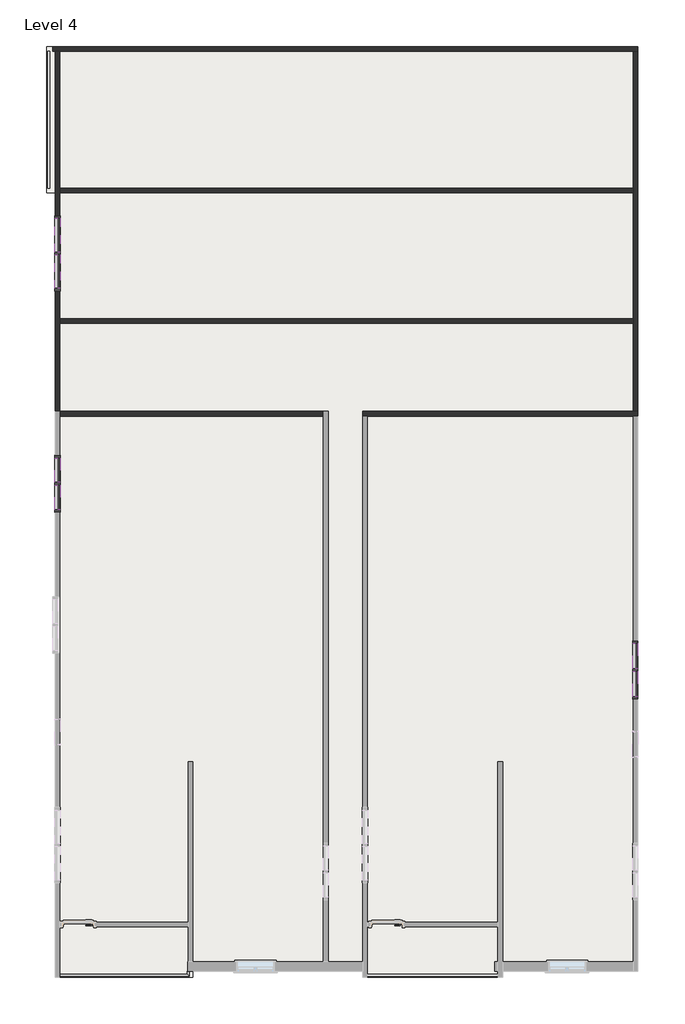
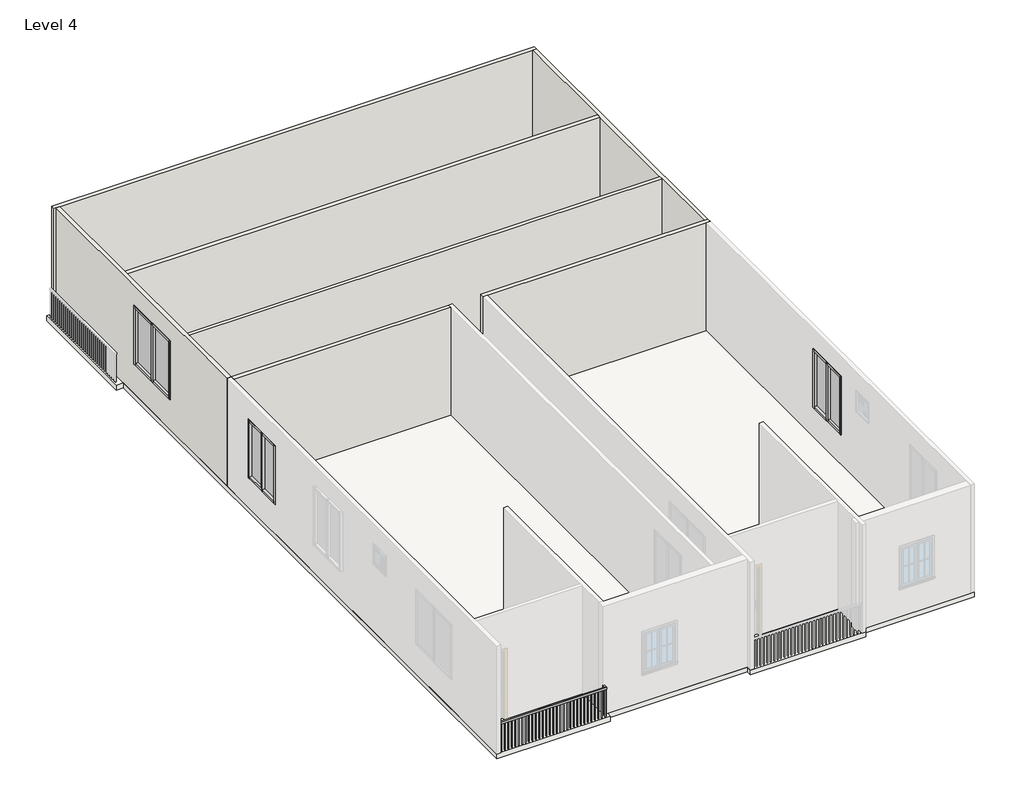
# One storey, part 2 of 3: 21 members, 7 walls, 6 plates, 1 railing, 1 slab.
"""IFC4 building model written with IfcOpenShell, lengths in millimetres."""

from ifc_helpers import new_model, si_unit, frame, origin, place, context, project, spatial, polyline, outline, extrude, faceted_brep, transform, mapped, element, save
from components import member_3f0e0172, member_96ae0c19, member_d60e8053, member_2fae0574, member_3e1d4a65, system_panel_glazed_c4393626, system_panel_glazed_d2c73f4b, system_panel_glazed_30879ba3

model = new_model("IFC4")

# Units and contexts
model_context = context("Model", 3, world=origin())
ifc_project = project(units=[si_unit("LENGTHUNIT", "METRE", prefix="MILLI")], contexts=[model_context])

# Site, building, storey
site = spatial("IfcSite", under=ifc_project)
building = spatial("IfcBuilding", under=site)
storey = spatial("IfcBuildingStorey", under=building, Name="Level 4", Elevation=10058.4)

# Members
placement = place(None, origin())
member_shape = member_3f0e0172(model_context)
element("IfcMember", 1, ObjectType="Rectangular Mullion : 2.5\" x 5\" rectangular", at=placement, inside=storey, context=model_context, shape_type="MappedRepresentation", body=[
    mapped(member_shape, transform((5848.1708786, -3933.7021821, 12801.6), x_axis=(0.0, 0.0, 1.0), y_axis=(-1.0, 0.0, 0.0), z_axis=(0.0, -1.0, 0.0))),
])
element("IfcMember", 2, ObjectType="Rectangular Mullion : 2.5\" x 5\" rectangular", at=placement, inside=storey, context=model_context, shape_type="MappedRepresentation", body=[
    mapped(member_shape, transform((5848.1708786, -3254.2521821, 12801.6), x_axis=(0.0, 0.0, 1.0), y_axis=(-1.0, 0.0, 0.0), z_axis=(0.0, -1.0, 0.0))),
])
element("IfcMember", 3, ObjectType="Rectangular Mullion : 2.5\" x 5\" rectangular", at=placement, inside=storey, context=model_context, shape_type="MappedRepresentation", body=[
    mapped(member_shape, transform((5848.1708786, -2638.3021821, 10972.8), x_axis=(0.0, 0.0, -1.0), y_axis=(-1.0, 0.0, 0.0), z_axis=(0.0, 1.0, 0.0))),
])
element("IfcMember", 4, ObjectType="Rectangular Mullion : 2.5\" x 5\" rectangular", at=placement, inside=storey, context=model_context, shape_type="MappedRepresentation", body=[
    mapped(member_shape, transform((5848.1708786, -3317.7521821, 10972.8), x_axis=(0.0, 0.0, -1.0), y_axis=(-1.0, 0.0, 0.0), z_axis=(0.0, 1.0, 0.0))),
])
member_2_shape = member_96ae0c19(model_context)
element("IfcMember", 5, ObjectType="Rectangular Mullion : 2.5\" x 5\" rectangular", at=placement, inside=storey, context=model_context, shape_type="MappedRepresentation", body=[
    mapped(member_2_shape, transform((-8153.157583, 600.1666267, 12801.6), x_axis=(0.0, 0.0, 1.0), y_axis=(-1.0, 0.0, 0.0), z_axis=(0.0, -1.0, 0.0))),
])
element("IfcMember", 6, ObjectType="Rectangular Mullion : 2.5\" x 5\" rectangular", at=placement, inside=storey, context=model_context, shape_type="MappedRepresentation", body=[
    mapped(member_2_shape, transform((-8153.157583, 1254.9937905, 12801.6), x_axis=(0.0, 0.0, 1.0), y_axis=(-1.0, 0.0, 0.0), z_axis=(0.0, -1.0, 0.0))),
])
element("IfcMember", 7, ObjectType="Rectangular Mullion : 2.5\" x 5\" rectangular", at=placement, inside=storey, context=model_context, shape_type="MappedRepresentation", body=[
    mapped(member_2_shape, transform((-8153.157583, 1846.3209543, 10972.8), x_axis=(0.0, 0.0, -1.0), y_axis=(-1.0, 0.0, 0.0), z_axis=(0.0, 1.0, 0.0))),
])
element("IfcMember", 8, ObjectType="Rectangular Mullion : 2.5\" x 5\" rectangular", at=placement, inside=storey, context=model_context, shape_type="MappedRepresentation", body=[
    mapped(member_2_shape, transform((-8153.157583, 1191.4937905, 10972.8), x_axis=(0.0, 0.0, -1.0), y_axis=(-1.0, 0.0, 0.0), z_axis=(0.0, 1.0, 0.0))),
])
member_3_shape = member_d60e8053(model_context)
element("IfcMember", 9, ObjectType="Rectangular Mullion : 2.5\" x 5\" rectangular", at=placement, inside=storey, context=model_context, shape_type="MappedRepresentation", body=[
    mapped(member_3_shape, transform((5848.1708786, -3286.0021821, 10972.8), x_axis=(0.0, -1.0, 0.0), y_axis=(-1.0, 0.0, 0.0), z_axis=(0.0, 0.0, -1.0))),
])
element("IfcMember", 10, ObjectType="Rectangular Mullion : 2.5\" x 5\" rectangular", at=placement, inside=storey, context=model_context, shape_type="MappedRepresentation", body=[
    mapped(member_3_shape, transform((-8153.157583, 1223.2437905, 10972.8), x_axis=(0.0, -1.0, 0.0), y_axis=(-1.0, 0.0, 0.0), z_axis=(0.0, 0.0, -1.0))),
])
element("IfcMember", 11, ObjectType="Rectangular Mullion : 2.5\" x 5\" rectangular", at=placement, inside=storey, context=model_context, shape_type="MappedRepresentation", body=[
    mapped(member_3_shape, transform((-8153.157583, 6807.1511393, 10972.8), x_axis=(0.0, -1.0, 0.0), y_axis=(-1.0, 0.0, 0.0), z_axis=(0.0, 0.0, -1.0))),
])
member_4_shape = member_2fae0574(model_context)
element("IfcMember", 12, ObjectType="Rectangular Mullion : 2.5\" x 5\" rectangular", at=placement, inside=storey, context=model_context, shape_type="MappedRepresentation", body=[
    mapped(member_4_shape, transform((5848.1708786, -2574.8021821, 12801.6), x_axis=(0.0, 1.0, 0.0), y_axis=(-1.0, 0.0, 0.0), z_axis=(0.0, 0.0, 1.0))),
])
element("IfcMember", 13, ObjectType="Rectangular Mullion : 2.5\" x 5\" rectangular", at=placement, inside=storey, context=model_context, shape_type="MappedRepresentation", body=[
    mapped(member_4_shape, transform((-8153.157583, 1909.8209543, 12801.6), x_axis=(0.0, 1.0, 0.0), y_axis=(-1.0, 0.0, 0.0), z_axis=(0.0, 0.0, 1.0))),
])
element("IfcMember", 14, ObjectType="Rectangular Mullion : 2.5\" x 5\" rectangular", at=placement, inside=storey, context=model_context, shape_type="MappedRepresentation", body=[
    mapped(member_4_shape, transform((-8153.157583, 7721.9533991, 12801.6), x_axis=(0.0, 1.0, 0.0), y_axis=(-1.0, 0.0, 0.0), z_axis=(0.0, 0.0, 1.0))),
])
element("IfcMember", 15, ObjectType="Rectangular Mullion : 2.5\" x 5\" rectangular", at=placement, inside=storey, context=model_context, shape_type="MappedRepresentation", body=[
    mapped(member_4_shape, transform((5848.1708786, -3997.2021821, 10972.8), x_axis=(0.0, -1.0, 0.0), y_axis=(-1.0, 0.0, 0.0), z_axis=(0.0, 0.0, -1.0))),
])
element("IfcMember", 16, ObjectType="Rectangular Mullion : 2.5\" x 5\" rectangular", at=placement, inside=storey, context=model_context, shape_type="MappedRepresentation", body=[
    mapped(member_4_shape, transform((-8153.157583, 536.6666267, 10972.8), x_axis=(0.0, -1.0, 0.0), y_axis=(-1.0, 0.0, 0.0), z_axis=(0.0, 0.0, -1.0))),
])
element("IfcMember", 17, ObjectType="Rectangular Mullion : 2.5\" x 5\" rectangular", at=placement, inside=storey, context=model_context, shape_type="MappedRepresentation", body=[
    mapped(member_4_shape, transform((-8153.157583, 5892.3488795, 10972.8), x_axis=(0.0, -1.0, 0.0), y_axis=(-1.0, 0.0, 0.0), z_axis=(0.0, 0.0, -1.0))),
])
member_5_shape = member_3e1d4a65(model_context)
element("IfcMember", 18, ObjectType="Rectangular Mullion : 2.5\" x 5\" rectangular", at=placement, inside=storey, context=model_context, shape_type="MappedRepresentation", body=[
    mapped(member_5_shape, transform((-8153.157583, 5955.8488795, 12801.6), x_axis=(0.0, 0.0, 1.0), y_axis=(-1.0, 0.0, 0.0), z_axis=(0.0, -1.0, 0.0))),
])
element("IfcMember", 19, ObjectType="Rectangular Mullion : 2.5\" x 5\" rectangular", at=placement, inside=storey, context=model_context, shape_type="MappedRepresentation", body=[
    mapped(member_5_shape, transform((-8153.157583, 6838.9011393, 12801.6), x_axis=(0.0, 0.0, 1.0), y_axis=(-1.0, 0.0, 0.0), z_axis=(0.0, -1.0, 0.0))),
])
element("IfcMember", 20, ObjectType="Rectangular Mullion : 2.5\" x 5\" rectangular", at=placement, inside=storey, context=model_context, shape_type="MappedRepresentation", body=[
    mapped(member_5_shape, transform((-8153.157583, 7658.4533991, 10972.8), x_axis=(0.0, 0.0, -1.0), y_axis=(-1.0, 0.0, 0.0), z_axis=(0.0, 1.0, 0.0))),
])
element("IfcMember", 21, ObjectType="Rectangular Mullion : 2.5\" x 5\" rectangular", at=placement, inside=storey, context=model_context, shape_type="MappedRepresentation", body=[
    mapped(member_5_shape, transform((-8153.157583, 6775.4011393, 10972.8), x_axis=(0.0, 0.0, -1.0), y_axis=(-1.0, 0.0, 0.0), z_axis=(0.0, 1.0, 0.0))),
])

# Plates
system_panel_glazed_shape = system_panel_glazed_c4393626(model_context)
element("IfcPlate", 22, ObjectType="System Panel : Glazed", at=placement, inside=storey, context=model_context, shape_type="MappedRepresentation", body=[
    mapped(system_panel_glazed_shape, transform((-8153.157583, 1550.6573724, 11036.3), x_axis=(0.0, -1.0, 0.0), y_axis=(1.0, 0.0, 0.0), z_axis=(0.0, 0.0, 1.0))),
])
element("IfcPlate", 23, ObjectType="System Panel : Glazed", at=placement, inside=storey, context=model_context, shape_type="MappedRepresentation", body=[
    mapped(system_panel_glazed_shape, transform((-8153.157583, 895.8302086, 11036.3), x_axis=(0.0, -1.0, 0.0), y_axis=(1.0, 0.0, 0.0), z_axis=(0.0, 0.0, 1.0))),
])
system_panel_glazed_2_shape = system_panel_glazed_d2c73f4b(model_context)
element("IfcPlate", 24, ObjectType="System Panel : Glazed", at=placement, inside=storey, context=model_context, shape_type="MappedRepresentation", body=[
    mapped(system_panel_glazed_2_shape, transform((5848.1708786, -2946.2771821, 11036.3), x_axis=(0.0, -1.0, 0.0), y_axis=(1.0, 0.0, 0.0), z_axis=(0.0, 0.0, 1.0))),
])
element("IfcPlate", 25, ObjectType="System Panel : Glazed", at=placement, inside=storey, context=model_context, shape_type="MappedRepresentation", body=[
    mapped(system_panel_glazed_2_shape, transform((5848.1708786, -3625.7271821, 11036.3), x_axis=(0.0, -1.0, 0.0), y_axis=(1.0, 0.0, 0.0), z_axis=(0.0, 0.0, 1.0))),
])
system_panel_glazed_3_shape = system_panel_glazed_30879ba3(model_context)
element("IfcPlate", 26, ObjectType="System Panel : Glazed", at=placement, inside=storey, context=model_context, shape_type="MappedRepresentation", body=[
    mapped(system_panel_glazed_3_shape, transform((-8153.157583, 7248.6772692, 11036.3), x_axis=(0.0, -1.0, 0.0), y_axis=(1.0, 0.0, 0.0), z_axis=(0.0, 0.0, 1.0))),
])
element("IfcPlate", 27, ObjectType="System Panel : Glazed", at=placement, inside=storey, context=model_context, shape_type="MappedRepresentation", body=[
    mapped(system_panel_glazed_3_shape, transform((-8153.157583, 6365.6250094, 11036.3), x_axis=(0.0, -1.0, 0.0), y_axis=(1.0, 0.0, 0.0), z_axis=(0.0, 0.0, 1.0))),
])

# Railing
element("IfcRailing", 28, ObjectType="Handrail - Rectangular", at=placement, inside=storey, context=model_context, shape_type="SolidModel", body=[
    faceted_brep([(-8153.157583, -10659.0005933, 10972.8), (-8153.157583, -10659.0005933, 10922.0), (-8153.157583, -10709.8005933, 10922.0), (-8153.157583, -10709.8005933, 10972.8), (-5014.0237038, -10659.0005933, 10972.8), (-5014.0237038, -10659.0005933, 10922.0), (-4963.2237038, -10709.8005933, 10922.0), (-4963.2237038, -10709.8005933, 10972.8), (-5014.0237038, -10582.0742041, 10972.8), (-4963.2237038, -10582.0742041, 10972.8), (-4963.2237038, -10582.0742041, 10922.0), (-5014.0237038, -10582.0742041, 10922.0)], [[[0, 1, 2, 3]], [[1, 0, 4, 5]], [[2, 1, 5, 6]], [[3, 2, 6, 7]], [[0, 3, 7, 4]], [[8, 9, 10, 11]], [[5, 4, 8, 11]], [[6, 5, 11, 10]], [[7, 6, 10, 9]], [[4, 7, 9, 8]]]),
    extrude(outline(polyline([(-4979.0987038, -10592.3255933), (-4998.1487038, -10592.3255933), (-4998.1487038, -10573.2755933), (-4979.0987038, -10573.2755933), (-4979.0987038, -10592.3255933)])), frame((0.0, 0.0, 10058.4), z_axis=(0.0, 0.0, 1.0), x_axis=(1.0, 0.0, 0.0)), (0.0, 0.0, 1.0), 863.6),
    extrude(outline(polyline([(-5013.082583, -10693.9255933), (-5013.082583, -10674.8755933), (-4994.032583, -10674.8755933), (-4994.032583, -10693.9255933), (-5013.082583, -10693.9255933)])), frame((0.0, 0.0, 10058.4), z_axis=(0.0, 0.0, 1.0), x_axis=(1.0, 0.0, 0.0)), (0.0, 0.0, 1.0), 863.6),
    extrude(outline(polyline([(-5114.682583, -10693.9255933), (-5114.682583, -10674.8755933), (-5095.632583, -10674.8755933), (-5095.632583, -10693.9255933), (-5114.682583, -10693.9255933)])), frame((0.0, 0.0, 10058.4), z_axis=(0.0, 0.0, 1.0), x_axis=(1.0, 0.0, 0.0)), (0.0, 0.0, 1.0), 863.6),
    extrude(outline(polyline([(-5216.282583, -10693.9255933), (-5216.282583, -10674.8755933), (-5197.232583, -10674.8755933), (-5197.232583, -10693.9255933), (-5216.282583, -10693.9255933)])), frame((0.0, 0.0, 10058.4), z_axis=(0.0, 0.0, 1.0), x_axis=(1.0, 0.0, 0.0)), (0.0, 0.0, 1.0), 863.6),
    extrude(outline(polyline([(-5317.882583, -10693.9255933), (-5317.882583, -10674.8755933), (-5298.832583, -10674.8755933), (-5298.832583, -10693.9255933), (-5317.882583, -10693.9255933)])), frame((0.0, 0.0, 10058.4), z_axis=(0.0, 0.0, 1.0), x_axis=(1.0, 0.0, 0.0)), (0.0, 0.0, 1.0), 863.6),
    extrude(outline(polyline([(-5419.482583, -10693.9255933), (-5419.482583, -10674.8755933), (-5400.432583, -10674.8755933), (-5400.432583, -10693.9255933), (-5419.482583, -10693.9255933)])), frame((0.0, 0.0, 10058.4), z_axis=(0.0, 0.0, 1.0), x_axis=(1.0, 0.0, 0.0)), (0.0, 0.0, 1.0), 863.6),
    extrude(outline(polyline([(-5521.082583, -10693.9255933), (-5521.082583, -10674.8755933), (-5502.032583, -10674.8755933), (-5502.032583, -10693.9255933), (-5521.082583, -10693.9255933)])), frame((0.0, 0.0, 10058.4), z_axis=(0.0, 0.0, 1.0), x_axis=(1.0, 0.0, 0.0)), (0.0, 0.0, 1.0), 863.6),
    extrude(outline(polyline([(-5622.682583, -10693.9255933), (-5622.682583, -10674.8755933), (-5603.632583, -10674.8755933), (-5603.632583, -10693.9255933), (-5622.682583, -10693.9255933)])), frame((0.0, 0.0, 10058.4), z_axis=(0.0, 0.0, 1.0), x_axis=(1.0, 0.0, 0.0)), (0.0, 0.0, 1.0), 863.6),
    extrude(outline(polyline([(-5724.282583, -10693.9255933), (-5724.282583, -10674.8755933), (-5705.232583, -10674.8755933), (-5705.232583, -10693.9255933), (-5724.282583, -10693.9255933)])), frame((0.0, 0.0, 10058.4), z_axis=(0.0, 0.0, 1.0), x_axis=(1.0, 0.0, 0.0)), (0.0, 0.0, 1.0), 863.6),
    extrude(outline(polyline([(-5825.882583, -10693.9255933), (-5825.882583, -10674.8755933), (-5806.832583, -10674.8755933), (-5806.832583, -10693.9255933), (-5825.882583, -10693.9255933)])), frame((0.0, 0.0, 10058.4), z_axis=(0.0, 0.0, 1.0), x_axis=(1.0, 0.0, 0.0)), (0.0, 0.0, 1.0), 863.6),
    extrude(outline(polyline([(-5927.482583, -10693.9255933), (-5927.482583, -10674.8755933), (-5908.432583, -10674.8755933), (-5908.432583, -10693.9255933), (-5927.482583, -10693.9255933)])), frame((0.0, 0.0, 10058.4), z_axis=(0.0, 0.0, 1.0), x_axis=(1.0, 0.0, 0.0)), (0.0, 0.0, 1.0), 863.6),
    extrude(outline(polyline([(-6029.082583, -10693.9255933), (-6029.082583, -10674.8755933), (-6010.032583, -10674.8755933), (-6010.032583, -10693.9255933), (-6029.082583, -10693.9255933)])), frame((0.0, 0.0, 10058.4), z_axis=(0.0, 0.0, 1.0), x_axis=(1.0, 0.0, 0.0)), (0.0, 0.0, 1.0), 863.6),
    extrude(outline(polyline([(-6130.682583, -10693.9255933), (-6130.682583, -10674.8755933), (-6111.632583, -10674.8755933), (-6111.632583, -10693.9255933), (-6130.682583, -10693.9255933)])), frame((0.0, 0.0, 10058.4), z_axis=(0.0, 0.0, 1.0), x_axis=(1.0, 0.0, 0.0)), (0.0, 0.0, 1.0), 863.6),
    extrude(outline(polyline([(-6232.282583, -10693.9255933), (-6232.282583, -10674.8755933), (-6213.232583, -10674.8755933), (-6213.232583, -10693.9255933), (-6232.282583, -10693.9255933)])), frame((0.0, 0.0, 10058.4), z_axis=(0.0, 0.0, 1.0), x_axis=(1.0, 0.0, 0.0)), (0.0, 0.0, 1.0), 863.6),
    extrude(outline(polyline([(-6333.882583, -10693.9255933), (-6333.882583, -10674.8755933), (-6314.832583, -10674.8755933), (-6314.832583, -10693.9255933), (-6333.882583, -10693.9255933)])), frame((0.0, 0.0, 10058.4), z_axis=(0.0, 0.0, 1.0), x_axis=(1.0, 0.0, 0.0)), (0.0, 0.0, 1.0), 863.6),
    extrude(outline(polyline([(-6435.482583, -10693.9255933), (-6435.482583, -10674.8755933), (-6416.432583, -10674.8755933), (-6416.432583, -10693.9255933), (-6435.482583, -10693.9255933)])), frame((0.0, 0.0, 10058.4), z_axis=(0.0, 0.0, 1.0), x_axis=(1.0, 0.0, 0.0)), (0.0, 0.0, 1.0), 863.6),
    extrude(outline(polyline([(-6537.082583, -10693.9255933), (-6537.082583, -10674.8755933), (-6518.032583, -10674.8755933), (-6518.032583, -10693.9255933), (-6537.082583, -10693.9255933)])), frame((0.0, 0.0, 10058.4), z_axis=(0.0, 0.0, 1.0), x_axis=(1.0, 0.0, 0.0)), (0.0, 0.0, 1.0), 863.6),
    extrude(outline(polyline([(-6638.682583, -10693.9255933), (-6638.682583, -10674.8755933), (-6619.632583, -10674.8755933), (-6619.632583, -10693.9255933), (-6638.682583, -10693.9255933)])), frame((0.0, 0.0, 10058.4), z_axis=(0.0, 0.0, 1.0), x_axis=(1.0, 0.0, 0.0)), (0.0, 0.0, 1.0), 863.6),
    extrude(outline(polyline([(-6740.282583, -10693.9255933), (-6740.282583, -10674.8755933), (-6721.232583, -10674.8755933), (-6721.232583, -10693.9255933), (-6740.282583, -10693.9255933)])), frame((0.0, 0.0, 10058.4), z_axis=(0.0, 0.0, 1.0), x_axis=(1.0, 0.0, 0.0)), (0.0, 0.0, 1.0), 863.6),
    extrude(outline(polyline([(-6841.882583, -10693.9255933), (-6841.882583, -10674.8755933), (-6822.832583, -10674.8755933), (-6822.832583, -10693.9255933), (-6841.882583, -10693.9255933)])), frame((0.0, 0.0, 10058.4), z_axis=(0.0, 0.0, 1.0), x_axis=(1.0, 0.0, 0.0)), (0.0, 0.0, 1.0), 863.6),
    extrude(outline(polyline([(-6943.482583, -10693.9255933), (-6943.482583, -10674.8755933), (-6924.432583, -10674.8755933), (-6924.432583, -10693.9255933), (-6943.482583, -10693.9255933)])), frame((0.0, 0.0, 10058.4), z_axis=(0.0, 0.0, 1.0), x_axis=(1.0, 0.0, 0.0)), (0.0, 0.0, 1.0), 863.6),
    extrude(outline(polyline([(-7045.082583, -10693.9255933), (-7045.082583, -10674.8755933), (-7026.032583, -10674.8755933), (-7026.032583, -10693.9255933), (-7045.082583, -10693.9255933)])), frame((0.0, 0.0, 10058.4), z_axis=(0.0, 0.0, 1.0), x_axis=(1.0, 0.0, 0.0)), (0.0, 0.0, 1.0), 863.6),
    extrude(outline(polyline([(-7146.682583, -10693.9255933), (-7146.682583, -10674.8755933), (-7127.632583, -10674.8755933), (-7127.632583, -10693.9255933), (-7146.682583, -10693.9255933)])), frame((0.0, 0.0, 10058.4), z_axis=(0.0, 0.0, 1.0), x_axis=(1.0, 0.0, 0.0)), (0.0, 0.0, 1.0), 863.6),
    extrude(outline(polyline([(-7248.282583, -10693.9255933), (-7248.282583, -10674.8755933), (-7229.232583, -10674.8755933), (-7229.232583, -10693.9255933), (-7248.282583, -10693.9255933)])), frame((0.0, 0.0, 10058.4), z_axis=(0.0, 0.0, 1.0), x_axis=(1.0, 0.0, 0.0)), (0.0, 0.0, 1.0), 863.6),
    extrude(outline(polyline([(-7349.882583, -10693.9255933), (-7349.882583, -10674.8755933), (-7330.832583, -10674.8755933), (-7330.832583, -10693.9255933), (-7349.882583, -10693.9255933)])), frame((0.0, 0.0, 10058.4), z_axis=(0.0, 0.0, 1.0), x_axis=(1.0, 0.0, 0.0)), (0.0, 0.0, 1.0), 863.6),
    extrude(outline(polyline([(-7451.482583, -10693.9255933), (-7451.482583, -10674.8755933), (-7432.432583, -10674.8755933), (-7432.432583, -10693.9255933), (-7451.482583, -10693.9255933)])), frame((0.0, 0.0, 10058.4), z_axis=(0.0, 0.0, 1.0), x_axis=(1.0, 0.0, 0.0)), (0.0, 0.0, 1.0), 863.6),
    extrude(outline(polyline([(-7553.082583, -10693.9255933), (-7553.082583, -10674.8755933), (-7534.032583, -10674.8755933), (-7534.032583, -10693.9255933), (-7553.082583, -10693.9255933)])), frame((0.0, 0.0, 10058.4), z_axis=(0.0, 0.0, 1.0), x_axis=(1.0, 0.0, 0.0)), (0.0, 0.0, 1.0), 863.6),
    extrude(outline(polyline([(-7654.682583, -10693.9255933), (-7654.682583, -10674.8755933), (-7635.632583, -10674.8755933), (-7635.632583, -10693.9255933), (-7654.682583, -10693.9255933)])), frame((0.0, 0.0, 10058.4), z_axis=(0.0, 0.0, 1.0), x_axis=(1.0, 0.0, 0.0)), (0.0, 0.0, 1.0), 863.6),
    extrude(outline(polyline([(-7756.282583, -10693.9255933), (-7756.282583, -10674.8755933), (-7737.232583, -10674.8755933), (-7737.232583, -10693.9255933), (-7756.282583, -10693.9255933)])), frame((0.0, 0.0, 10058.4), z_axis=(0.0, 0.0, 1.0), x_axis=(1.0, 0.0, 0.0)), (0.0, 0.0, 1.0), 863.6),
    extrude(outline(polyline([(-7857.882583, -10693.9255933), (-7857.882583, -10674.8755933), (-7838.832583, -10674.8755933), (-7838.832583, -10693.9255933), (-7857.882583, -10693.9255933)])), frame((0.0, 0.0, 10058.4), z_axis=(0.0, 0.0, 1.0), x_axis=(1.0, 0.0, 0.0)), (0.0, 0.0, 1.0), 863.6),
    extrude(outline(polyline([(-7959.482583, -10693.9255933), (-7959.482583, -10674.8755933), (-7940.432583, -10674.8755933), (-7940.432583, -10693.9255933), (-7959.482583, -10693.9255933)])), frame((0.0, 0.0, 10058.4), z_axis=(0.0, 0.0, 1.0), x_axis=(1.0, 0.0, 0.0)), (0.0, 0.0, 1.0), 863.6),
    extrude(outline(polyline([(-8061.082583, -10693.9255933), (-8061.082583, -10674.8755933), (-8042.032583, -10674.8755933), (-8042.032583, -10693.9255933), (-8061.082583, -10693.9255933)])), frame((0.0, 0.0, 10058.4), z_axis=(0.0, 0.0, 1.0), x_axis=(1.0, 0.0, 0.0)), (0.0, 0.0, 1.0), 863.6),
    extrude(outline(polyline([(-4998.1487038, -10693.9255933), (-4998.1487038, -10674.8755933), (-4979.0987038, -10674.8755933), (-4979.0987038, -10693.9255933), (-4998.1487038, -10693.9255933)])), frame((0.0, 0.0, 10058.4), z_axis=(0.0, 0.0, 1.0), x_axis=(1.0, 0.0, 0.0)), (0.0, 0.0, 1.0), 863.6),
    extrude(outline(polyline([(-4979.0987038, -10601.1242041), (-4998.1487038, -10601.1242041), (-4998.1487038, -10582.0742041), (-4979.0987038, -10582.0742041), (-4979.0987038, -10601.1242041)])), frame((0.0, 0.0, 10058.4), z_axis=(0.0, 0.0, 1.0), x_axis=(1.0, 0.0, 0.0)), (0.0, 0.0, 1.0), 863.6),
    extrude(outline(polyline([(-8153.157583, -10693.9255933), (-8153.157583, -10674.8755933), (-8134.107583, -10674.8755933), (-8134.107583, -10693.9255933), (-8153.157583, -10693.9255933)])), frame((0.0, 0.0, 10058.4), z_axis=(0.0, 0.0, 1.0), x_axis=(1.0, 0.0, 0.0)), (0.0, 0.0, 1.0), 863.6),
])

# Slab
element("IfcSlab", 29, ObjectType="6\" floor", at=placement, inside=storey, context=model_context, shape_type="SweptSolid", body=[
    extrude(outline(polyline([(5905.3208786, 11818.2189683), (5905.3208786, -10585.8779557), (2630.290751, -10585.8779557), (2630.290751, -10737.6531157), (-762.8431282, -10737.6531157), (-762.8431282, -10585.8779557), (-4874.3237038, -10585.8779557), (-4874.3237038, -10733.8493641), (-8210.307583, -10733.8493641), (-8210.307583, 8277.3011327), (-8419.607647, 8277.3011327), (-8419.607647, 11818.2189683), (5905.3208786, 11818.2189683)])), frame((0.0, 0.0, 9906.0), z_axis=(0.0, 0.0, 1.0), x_axis=(1.0, 0.0, 0.0)), (0.0, 0.0, 1.0), 152.4),
])

# Walls
element("IfcWall", 30, ObjectType="4.5\" wall", at=placement, inside=storey, context=model_context, shape_type="Brep", body=[
    faceted_brep([(-8267.457583, 11703.9189683, 10058.4), (-8210.307583, 11703.9189683, 10058.4), (-8096.007583, 11703.9189683, 10058.4), (5791.0208786, 11703.9189683, 10058.4), (5905.3208786, 11703.9189683, 10058.4), (5905.3208786, 11703.9189683, 13411.2), (5791.0208786, 11703.9189683, 13411.2), (-8096.007583, 11703.9189683, 13411.2), (-8210.307583, 11703.9189683, 13411.2), (-8267.457583, 11703.9189683, 13411.2), (-8267.457583, 11818.2189683, 10058.4), (-8267.457583, 11818.2189683, 13411.2), (5905.3208786, 11818.2189683, 13411.2), (5905.3208786, 11818.2189683, 10058.4)], [[[0, 1, 2, 3, 4, 5, 6, 7, 8, 9]], [[10, 11, 12, 13]], [[4, 3, 2, 1, 0, 10, 13]], [[9, 8, 7, 6, 5, 12, 11]], [[0, 9, 11, 10]], [[5, 4, 13, 12]]]),
])
element("IfcWall", 31, ObjectType="4.5\" wall", at=placement, inside=storey, context=model_context, shape_type="Brep", body=[
    faceted_brep([(5791.0208786, 11703.9189683, 10058.4), (5791.0208786, 8387.4224771, 10058.4), (5791.0208786, 8273.1224771, 10058.4), (5791.0208786, 5226.5048975, 10058.4), (5791.0208786, 5112.2048975, 10058.4), (5791.0208786, 2978.3002499, 10058.4), (5791.0208786, 2978.3002499, 13411.2), (5791.0208786, 5112.2048975, 13411.2), (5791.0208786, 5226.5048975, 13411.2), (5791.0208786, 8273.1224771, 13411.2), (5791.0208786, 8387.4224771, 13411.2), (5791.0208786, 11703.9189683, 13411.2), (5905.3208786, 11703.9189683, 10058.4), (5905.3208786, 11703.9189683, 13411.2), (5905.3208786, 2978.3002499, 13411.2), (5905.3208786, 2978.3002499, 10058.4)], [[[0, 1, 2, 3, 4, 5, 6, 7, 8, 9, 10, 11]], [[12, 13, 14, 15]], [[5, 4, 3, 2, 1, 0, 12, 15]], [[11, 10, 9, 8, 7, 6, 14, 13]], [[0, 11, 13, 12]], [[6, 5, 15, 14]]]),
])
element("IfcWall", 32, ObjectType="4.5\" wall", at=placement, inside=storey, context=model_context, shape_type="SweptSolid", body=[
    extrude(outline(polyline([(-1713.5935762, 2864.0002499), (-8096.007583, 2864.0002499), (-8096.007583, 2978.3002499), (-1713.5935762, 2978.3002499), (-1713.5935762, 2864.0002499)])), frame((0.0, 0.0, 10058.4), z_axis=(0.0, 0.0, 1.0), x_axis=(1.0, 0.0, 0.0)), (0.0, 0.0, 1.0), 3352.8),
])
element("IfcWall", 33, ObjectType="4.5\" wall", at=placement, inside=storey, context=model_context, shape_type="SweptSolid", body=[
    extrude(outline(polyline([(-8096.007583, 5226.5048975), (5791.0208786, 5226.5048975), (5791.0208786, 5112.2048975), (-8096.007583, 5112.2048975), (-8096.007583, 5226.5048975)])), frame((0.0, 0.0, 10058.4), z_axis=(0.0, 0.0, 1.0), x_axis=(1.0, 0.0, 0.0)), (0.0, 0.0, 1.0), 3352.8),
])
element("IfcWall", 34, ObjectType="4.5\" wall", at=placement, inside=storey, context=model_context, shape_type="SweptSolid", body=[
    extrude(outline(polyline([(-8096.007583, 8387.4224771), (5791.0208786, 8387.4224771), (5791.0208786, 8273.1224771), (-8096.007583, 8273.1224771), (-8096.007583, 8387.4224771)])), frame((0.0, 0.0, 10058.4), z_axis=(0.0, 0.0, 1.0), x_axis=(1.0, 0.0, 0.0)), (0.0, 0.0, 1.0), 3352.8),
])
element("IfcWall", 35, ObjectType="4.5\" wall", at=placement, inside=storey, context=model_context, shape_type="Brep", body=[
    faceted_brep([(-8096.007583, 2978.3002499, 10058.4), (-8096.007583, 5112.2048975, 10058.4), (-8096.007583, 5226.5048975, 10058.4), (-8096.007583, 8273.1224771, 10058.4), (-8096.007583, 8387.4224771, 10058.4), (-8096.007583, 11703.9189683, 10058.4), (-8096.007583, 11703.9189683, 13411.2), (-8096.007583, 8387.4224771, 13411.2), (-8096.007583, 8273.1224771, 13411.2), (-8096.007583, 5226.5048975, 13411.2), (-8096.007583, 5112.2048975, 13411.2), (-8096.007583, 2978.3002499, 13411.2), (-8096.007583, 7721.9533991, 12801.6), (-8096.007583, 7721.9533991, 10972.8), (-8096.007583, 5892.3488795, 10972.8), (-8096.007583, 5892.3488795, 12801.6), (-8210.307583, 11703.9189683, 10058.4), (-8210.307583, 2978.3002499, 10058.4), (-8210.307583, 2978.3002499, 13411.2), (-8210.307583, 11703.9189683, 13411.2), (-8210.307583, 7721.9533991, 10972.8), (-8210.307583, 7721.9533991, 12801.6), (-8210.307583, 5892.3488795, 12801.6), (-8210.307583, 5892.3488795, 10972.8)], [[[0, 1, 2, 3, 4, 5, 6, 7, 8, 9, 10, 11], [12, 13, 14, 15]], [[16, 17, 18, 19], [20, 21, 22, 23]], [[5, 4, 3, 2, 1, 0, 17, 16]], [[11, 10, 9, 8, 7, 6, 19, 18]], [[6, 5, 16, 19]], [[0, 11, 18, 17]], [[20, 13, 12, 21]], [[21, 12, 15, 22]], [[22, 15, 14, 23]], [[13, 20, 23, 14]]]),
])
element("IfcWall", 36, ObjectType="4.5\" wall", at=placement, inside=storey, context=model_context, shape_type="Brep", body=[
    faceted_brep([(-762.8431282, 2864.0002499, 10058.4), (-648.5431282, 2864.0002499, 10058.4), (5791.0208786, 2864.0002499, 10058.4), (5905.3208786, 2864.0002499, 10058.4), (5905.3208786, 2864.0002499, 13411.2), (5791.0208786, 2864.0002499, 13411.2), (-648.5431282, 2864.0002499, 13411.2), (-762.8431282, 2864.0002499, 13411.2), (-762.8431282, 2978.3002499, 10058.4), (-762.8431282, 2978.3002499, 13411.2), (5791.0208786, 2978.3002499, 13411.2), (5905.3208786, 2978.3002499, 13411.2), (5905.3208786, 2978.3002499, 10058.4), (5791.0208786, 2978.3002499, 10058.4)], [[[0, 1, 2, 3, 4, 5, 6, 7]], [[8, 9, 10, 11, 12, 13]], [[3, 2, 1, 0, 8, 13, 12]], [[7, 6, 5, 4, 11, 10, 9]], [[4, 3, 12, 11]], [[0, 7, 9, 8]]]),
])

save(model, "model.ifc")

# Revit data of these elements
# Type "Rectangular Mullion : 2.5\" x 5\" rectangular"
#   built-in parameter 1007304 = 0.416667 (stored number, unit not read)
#   built-in parameter 1007301 = 0.104167 (stored number, unit not read)
#   built-in parameter 1007300 = 0.104167 (stored number, unit not read)
# Type "System Panel : Glazed"
#   Construction Type Id = "GSP4R"
#   Analytic Construction = "1/8 in Pilkington single glazing"
#   Visual Light Transmittance = 0.9
#   Solar Heat Gain Coefficient = 0.86
#   Heat Transfer Coefficient (U) = 1.18115 BTU/(h·ft²·°F)
#   Define Thermal Properties by = 1
# Type "Handrail - Rectangular"
#   Assembly Code = "C2010400"
#   built-in parameter 1008612 = 0.0416667 (stored number, unit not read)
#   built-in parameter 1008611 = 0.0416667 (stored number, unit not read)
#   built-in parameter 1008609 = 0.333333 (stored number, unit not read)
#   built-in parameter 1008604 = 0.166667 (stored number, unit not read)
#   built-in parameter 1008603 = 0.166667 (stored number, unit not read)
#   Railing Height = 3' - 0"
#   built-in parameter 1008630 = 2
#   built-in parameter 1008610 = 2
#   built-in parameter 1008618 = Baluster - Square : 3/4"
# Type "6\" floor"
#   Assembly Code = "B1010"
#   Function = 0
#   Layers, outside or top first: 0' - 6" no material (function 1)
# Type "4.5\" wall"
#   Assembly Code = "B2010"
#   Layers, outside or top first: 0' - 4 1/2" no material (function 1)
# Elements 1, 2, 3, 4, 5, 6, 7, 8, 9, 10, 11, 12, 13, 14, 15, 16, 17, 18, 19, 20, 21 (IfcMember, "Rectangular Mullion : 2.5\" x 5\" rectangular")
#   Phase Created = New Construction
#   Materials on its faces: "Aluminum"
# Elements 22, 23, 24, 25, 26, 27 (IfcPlate, "System Panel : Glazed")
#   Phase Created = New Construction
#   Materials on its faces: "Glass"
# Element 28 (IfcRailing, "Handrail - Rectangular")
#   Phase Created = New Construction
# Element 29 (IfcSlab, "6\" floor")
#   Height Offset From Level = 0' - 0"
#   Phase Created = New Construction
#   Materials on its faces: "Default Floor"
# Elements 30, 31, 32, 33, 34, 35, 36 (IfcWall, "4.5\" wall")
#   Top Offset = -1' - 6"
#   Base Offset = 0' - 0"
#   Unconnected Height = 11' - 0"
#   wall height = 11' - 0"
#   Phase Created = New Construction
#   Base Constraint = Level 4
#   Materials on its faces: "Default Wall"
# Materials
#   "Aluminum": class "Metal", colour RGB 247 247 247, transparency 0, Description = "Aluminum 6061", Cost = 0
#   "Glass": class "Glass", colour RGB 0 128 192, transparency 0.75, Description = "Soda Lime Glass", Cost = 0
#   "Default Floor": colour RGB 128 128 128, transparency 0, Cost = 0
#   "Default Wall": colour RGB 128 128 128, transparency 0, Cost = 0
